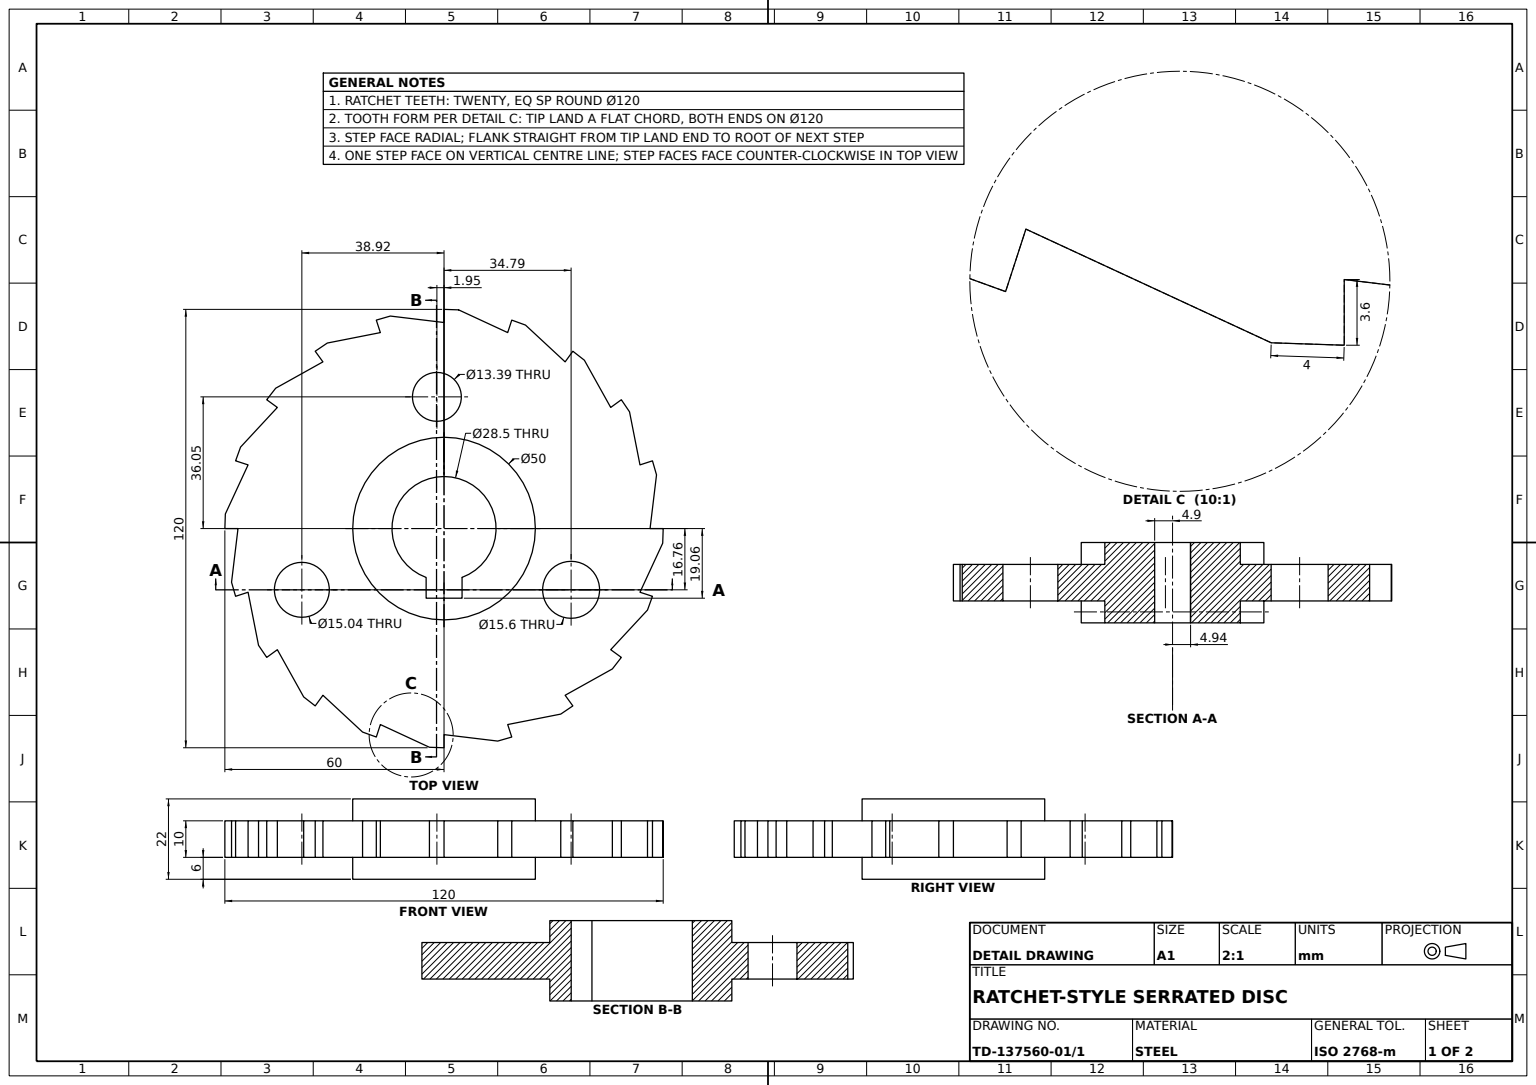
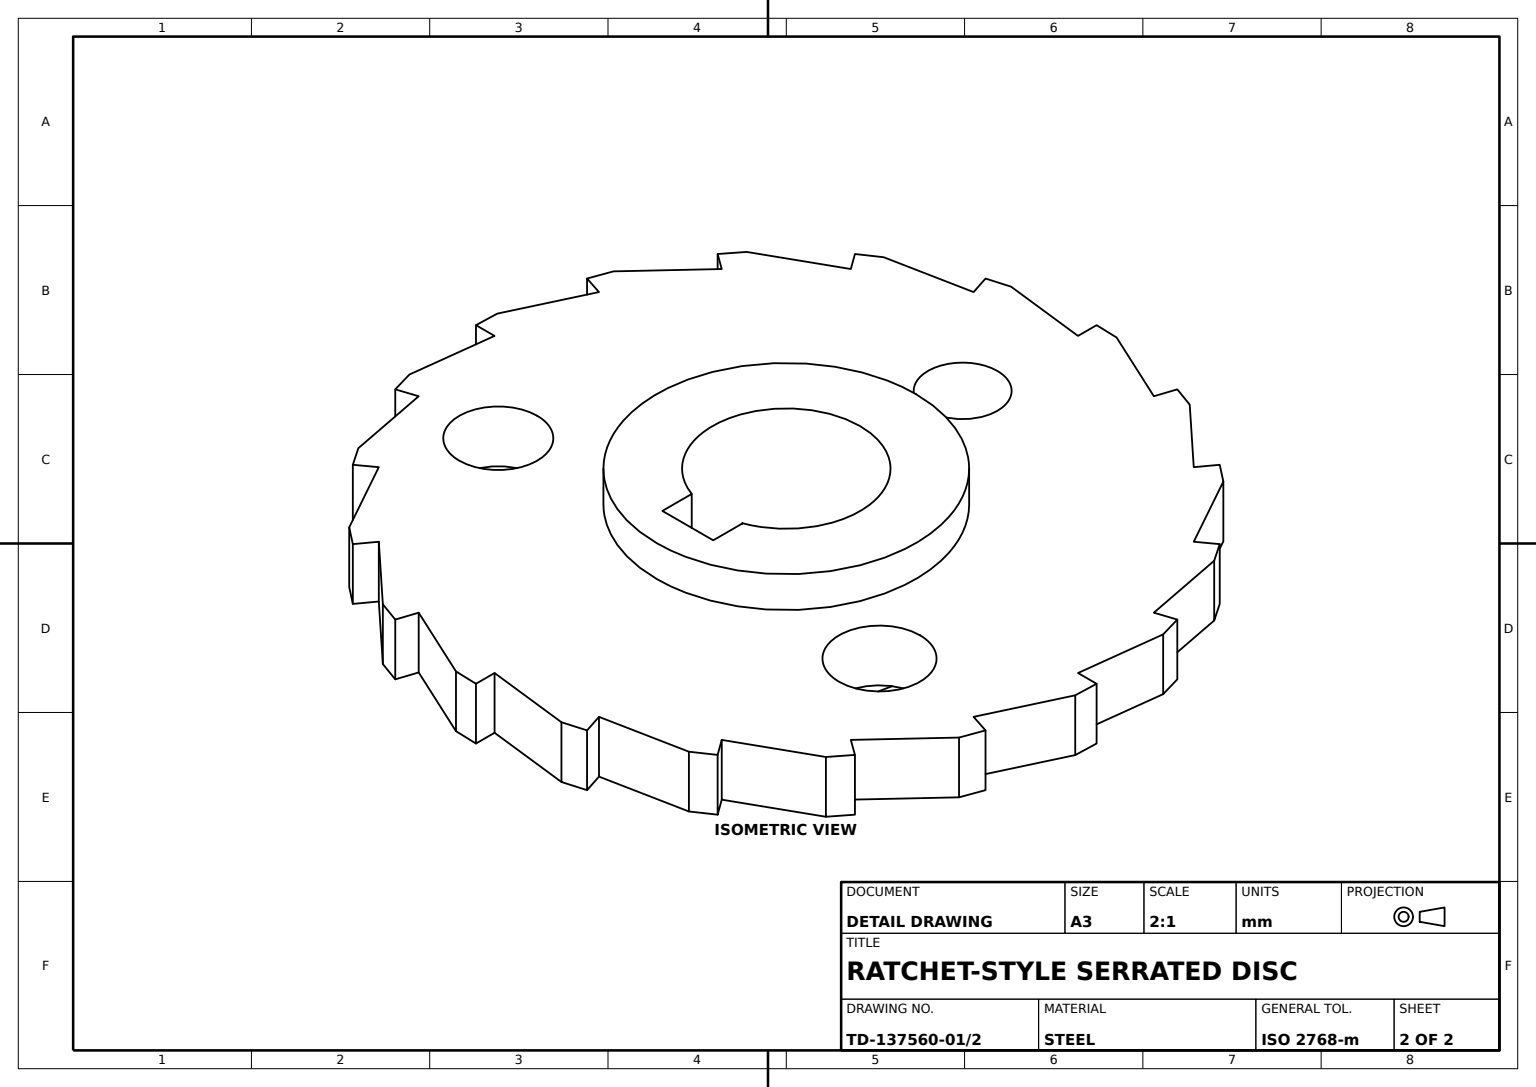
from build123d import *

# Parameters (mm, degrees)
RATCHET_WHEEL_BODY_20T_DEPTH = 10
HUB_BOSS_50_DEPTH            = 6
HUB_BOSS_50_DEPTH_BACK       = 16
HUB_SKETCH_R                 = 25
KEYED_SHAFT_BORE_DEPTH       = 57
THROUGH_HOLES_3X_DEPTH       = 57
THROUGH_HOLES_3X_DEPTH_BACK  = 57
THROUGH_HOLES_SKETCH_R       = 7.52194346
THROUGH_HOLES_SKETCH_R_2     = 7.800691594
THROUGH_HOLES_SKETCH_R_3     = 6.694831741


with BuildPart() as part:
    # Ratchet Tooth Profile Sketch → Ratchet Wheel Body 20T (new body)
    with BuildSketch(Plane(origin=(0, 0, 0), x_dir=(1, 0, 0), z_dir=(0, 1, 0))):
        Polygon((-14.697659706, -58.171976064), (0, -56.403789421), (0, -60), (3.997824162, -59.866663528), (17.429729478, -53.643191472), (18.541019662, -57.063390978), (22.301973147, -55.701184851), (23.837157922, -54.276602012), (33.153315595, -45.631624189), (35.267115138, -48.541019662), (38.423049613, -46.083286107), (45.631624189, -33.153315595), (48.541019662, -35.267115138), (50.783010274, -31.954434238), (53.643191472, -17.429729478), (57.063390978, -18.541019662), (58.171976064, -14.697659706), (56.403789421, 0), (60, 0), (59.866663528, 3.997824162), (53.643191472, 17.429729478), (57.063390978, 18.541019662), (55.701184851, 22.301973147), (45.631624189, 33.153315595), (48.541019662, 35.267115138), (46.083286107, 38.423049613), (33.153315595, 45.631624189), (35.267115138, 48.541019662), (31.954434238, 50.783010274), (17.429729478, 53.643191472), (18.541019662, 57.063390978), (14.697659706, 58.171976064), (0, 56.403789421), (0, 60), (-3.997824162, 59.866663528), (-17.429729478, 53.643191472), (-18.541019662, 57.063390978), (-22.301973147, 55.701184851), (-33.153315595, 45.631624189), (-35.267115138, 48.541019662), (-38.423049613, 46.083286107), (-45.631624189, 33.153315595), (-48.541019662, 35.267115138), (-50.783010274, 31.954434238), (-53.643191472, 17.429729478), (-57.063390978, 18.541019662), (-58.171976064, 14.697659706), (-56.403789421, 0), (-60, 0), (-59.866663528, -3.997824162), (-53.643191472, -17.429729478), (-57.063390978, -18.541019662), (-55.701184851, -22.301973147), (-45.631624189, -33.153315595), (-48.541019662, -35.267115138), (-46.083286107, -38.423049613), (-33.153315595, -45.631624189), (-35.267115138, -48.541019662), (-31.954434238, -50.783010274), (-17.429729478, -53.643191472), (-18.541019662, -57.063390978), align=None)
    extrude(amount=RATCHET_WHEEL_BODY_20T_DEPTH)

    # Hub Sketch → Hub Boss Ø50 (add, two sides: drawn at the far end of the back side and taken through both)
    with BuildSketch(Plane(origin=(0, 10, 0), x_dir=(1, 0, 0), z_dir=(0, 1, 0)).offset(-HUB_BOSS_50_DEPTH_BACK)):
        with Locations(Location((0, 0, 0), (0, 0, 270))):
            Circle(HUB_SKETCH_R)
    extrude(amount=HUB_BOSS_50_DEPTH + HUB_BOSS_50_DEPTH_BACK)

    # Keyed Bore Sketch → Keyed Shaft Bore (cut)
    with BuildSketch(Plane(origin=(0, 16, 0), x_dir=(1, 0, 0), z_dir=(0, 1, 0))):
        with BuildLine():
            Line((4.898606828, 13.381560116), (4.937062937, 13.381560116))
            Line((4.937062937, 13.381560116), (4.937062937, 19.059359245))
            Line((4.937062937, 19.059359245), (-4.898606828, 19.059359245))
            Line((-4.898606828, 19.059359245), (-4.898606828, 13.381560116))
            ThreePointArc((-4.898606828, 13.381560116), (0, -14.25), (4.898606828, 13.381560116))
        make_face()
    extrude(amount=-KEYED_SHAFT_BORE_DEPTH, mode=Mode.SUBTRACT)

    # Through Holes Sketch → Through Holes 3x (cut, two sides: drawn at the far end of the back side and taken through both)
    with BuildSketch(Plane(origin=(0, 0, 0), x_dir=(1, 0, 0), z_dir=(0, 1, 0)).offset(-THROUGH_HOLES_3X_DEPTH_BACK)):
        with Locations(Location((-38.922426411, 16.763050903, 0), (0, 0, 270))):
            Circle(THROUGH_HOLES_SKETCH_R)
        with Locations(Location((34.789071394, 16.763050903, 0), (0, 0, 270))):
            Circle(THROUGH_HOLES_SKETCH_R_2)
        with Locations(Location((-1.951862091, -36.052040982, 0), (0, 0, 270))):
            Circle(THROUGH_HOLES_SKETCH_R_3)
    extrude(amount=THROUGH_HOLES_3X_DEPTH + THROUGH_HOLES_3X_DEPTH_BACK, mode=Mode.SUBTRACT)


solid = part.part
